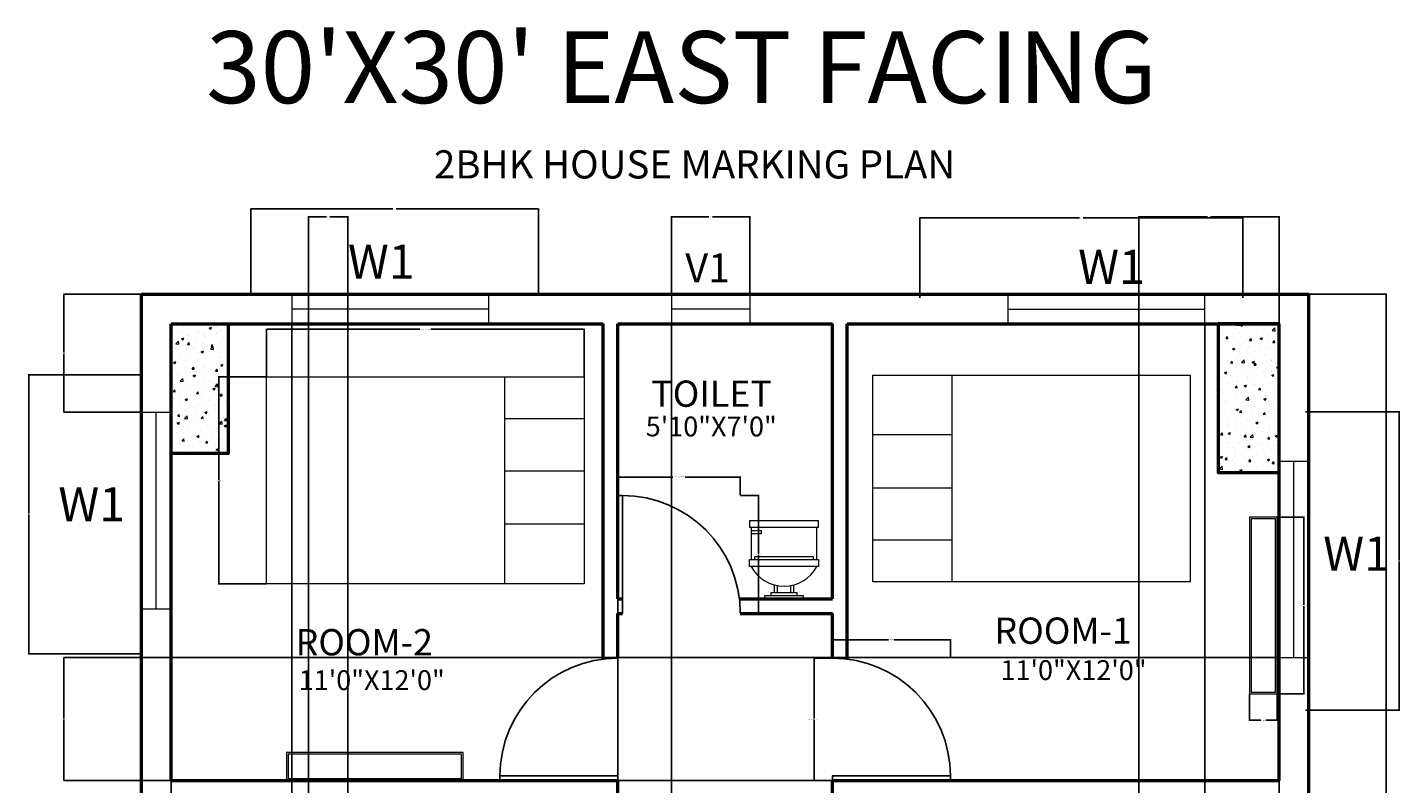
# Model space of a CAD drawing. Units: inches. Extents: x -26 to 394, y -29 to 465.
# Tile 2 of 2: x -25 to 394, y 234 to 465. Entities that reach past the tile are written whole.
import ezdxf

# ---------------------------------------------------------------- set-up
doc = ezdxf.new("R2010")
doc.units = ezdxf.units.IN
doc.header["$MEASUREMENT"] = 0
for name, color, linetype, lineweight, true_color in [('A-ANNO-DIMS', 254, 'Continuous', 18, 0xfeeab9), ('A-COLS', 254, 'Continuous', 50, 0xfeeab9), ('A-COLS-PATT', 31, 'Continuous', 13, 0xfecc66), ('A-FLOR-FIXT', 254, 'Continuous', 18, 0xfeeab9), ('A-FURN', 254, 'Continuous', 18, 0xfeeab9)]:
    doc.layers.add(name, color=color, linetype=linetype, lineweight=lineweight, true_color=true_color)
for name, color, linetype, lineweight in [('A-ANNO-TEXT', 7, 'Continuous', 18), ('A-ANNO-TTLB', 7, 'Continuous', 35), ('A-AREA-IDEN', 7, 'Continuous', 25), ('A-DOOR', 3, 'Continuous', 25), ('A-GLAZ', 4, 'Continuous', 18), ('A-WALL', 7, 'Continuous', 50)]:
    doc.layers.add(name, color=color, linetype=linetype, lineweight=lineweight)
doc.styles.get("Standard").update_dxf_attribs({"font": 'arial.ttf'})
doc.dimstyles.get("Standard").update_dxf_attribs({"dimtxt": 0.18, "dimasz": 0.18, "dimexe": 0.18, "dimexo": 0.0625, "dimgap": 0.09, "dimtad": 0, "dimtih": 1, "dimtoh": 1, "dimdec": 4, "dimzin": 0, "dimdsep": 46, "dimtxsty": 'Standard', "dimcen": 0.09, "dimadec": 0, "dimazin": 0, "dimtfac": 1, "dimtdec": 4, "dimtofl": 0, "dimtmove": 0, "dimatfit": 3, "dimfxl": 1, "dimtolj": 1, "dimtzin": 0, "dimarcsym": 0})

# ---------------------------------------------------------------- blocks, each defined once
blk = doc.blocks.new('*U5')
for p, q in [((-10, 22), (-10, 12)), ((-10, 21), (-7, 21)), ((-7, 21), (-7, 20)), ((10, 12), (10, 22)), ((-7, 20), (-10, 20)), ((9, 13), (-9, 13)), ((-9, 13), (-9, 12)), ((9, 12), (9, 13)), ((10.5, 12), (-10.5, 12)), ((-10.5, 10), (-10.5, 12)), ((10.5, 10), (-10.5, 10)), ((10.5, 12), (10.5, 10)), ((-3, 4.4065), (-3, 2)), ((3, 2), (3, 4.4065)), ((4, 2), (-4, 2)), ((-4, 2), (-4, 1)), ((-2, 2), (-2, 4.1658)), ((2, 4.1658), (2, 2)), ((4, 1), (4, 2))]:
    blk.add_line(p, q)
for points in [[(10.5, 22), (10.5, 24), (-10.5, 24), (-10.5, 22)], [(6, 0), (6, 1), (-6, 1), (-6, 0)]]:
    blk.add_lwpolyline(points, close=True)
blk.add_arc((0, 15.3333), 11.3333, 208.0725, 331.9275)
blk = doc.blocks.new('*D6')
at = {"layer": 'A-ANNO-DIMS', "color": 0, "lineweight": -2, "transparency": 16777216}
for p, q in [((9.23, 358.7), (-24.76, 358.7)), ((-24.58, 358.52), (-24.58, 316.25)), ((-24.58, 273.62), (-24.58, 315.89)), ((9.23, 273.44), (-24.76, 273.44))]:
    blk.add_line(p, q, dxfattribs=at)
at = {"layer": 'A-ANNO-DIMS', "color": 0, "transparency": 16777216}
for points in [[(-24.61, 358.52), (-24.55, 358.52), (-24.58, 358.7)], [(-24.61, 273.62), (-24.55, 273.62), (-24.58, 273.44)]]:
    blk.add_solid(points, dxfattribs=at)
at = {"layer": 'Defpoints', "color": 0, "transparency": 16777216}
for p in [(9.29, 358.7), (-24.58, 273.44), (9.29, 273.44)]:
    blk.add_point(p, dxfattribs=at)
at = {"layer": 'A-ANNO-DIMS', "color": 0, "transparency": 16777216, "insert": (-24.58, 316.07), "char_height": 0.18, "attachment_point": 5}
blk.add_mtext('\\A1;85.2658', dxfattribs=at)
blk = doc.blocks.new('*D7')
at = {"layer": 'A-ANNO-DIMS', "color": 0, "lineweight": -2, "transparency": 16777216}
for p, q in [((43.18, 382.82), (43.18, 409.48)), ((43.36, 409.3), (86.58, 409.3)), ((130.86, 409.3), (87.65, 409.3)), ((131.04, 382.82), (131.04, 409.48))]:
    blk.add_line(p, q, dxfattribs=at)
at = {"layer": 'A-ANNO-DIMS', "color": 0, "transparency": 16777216}
for points in [[(43.36, 409.33), (43.36, 409.27), (43.18, 409.3)], [(130.86, 409.33), (130.86, 409.27), (131.04, 409.3)]]:
    blk.add_solid(points, dxfattribs=at)
at = {"layer": 'Defpoints', "color": 0, "transparency": 16777216}
for p in [(131.04, 409.3), (43.18, 382.76), (131.04, 382.76)]:
    blk.add_point(p, dxfattribs=at)
at = {"layer": 'A-ANNO-DIMS', "color": 0, "transparency": 16777216, "insert": (87.11, 409.3), "char_height": 0.18, "attachment_point": 5}
blk.add_mtext('\\A1;87.8626', dxfattribs=at)
blk = doc.blocks.new('*D8')
at = {"layer": 'A-ANNO-DIMS', "color": 0, "lineweight": -2, "transparency": 16777216}
for p, q in [((247.51, 382.14), (247.51, 406.75)), ((247.69, 406.57), (296.36, 406.57)), ((346.09, 406.57), (297.43, 406.57)), ((346.27, 382.14), (346.27, 406.75))]:
    blk.add_line(p, q, dxfattribs=at)
at = {"layer": 'A-ANNO-DIMS', "color": 0, "transparency": 16777216}
for points in [[(247.69, 406.6), (247.69, 406.54), (247.51, 406.57)], [(346.09, 406.6), (346.09, 406.54), (346.27, 406.57)]]:
    blk.add_solid(points, dxfattribs=at)
at = {"layer": 'Defpoints', "color": 0, "transparency": 16777216}
for p in [(346.27, 406.57), (247.51, 382.08), (346.27, 382.08)]:
    blk.add_point(p, dxfattribs=at)
at = {"layer": 'A-ANNO-DIMS', "color": 0, "transparency": 16777216, "insert": (296.89, 406.57), "char_height": 0.18, "attachment_point": 5}
blk.add_mtext('\\A1;98.7602', dxfattribs=at)
blk = doc.blocks.new('*D9')
at = {"layer": 'A-ANNO-DIMS', "color": 0, "lineweight": -2, "transparency": 16777216}
for p, q in [((365.41, 347.37), (394.13, 347.37)), ((393.95, 347.19), (393.95, 301.96)), ((393.95, 256.37), (393.95, 301.6)), ((365.41, 256.19), (394.13, 256.19))]:
    blk.add_line(p, q, dxfattribs=at)
at = {"layer": 'A-ANNO-DIMS', "color": 0, "transparency": 16777216}
for points in [[(393.92, 347.19), (393.98, 347.19), (393.95, 347.37)], [(393.92, 256.37), (393.98, 256.37), (393.95, 256.19)]]:
    blk.add_solid(points, dxfattribs=at)
at = {"layer": 'Defpoints', "color": 0, "transparency": 16777216}
for p in [(365.34, 347.37), (365.34, 256.19), (393.95, 256.19)]:
    blk.add_point(p, dxfattribs=at)
at = {"layer": 'A-ANNO-DIMS', "color": 0, "transparency": 16777216, "insert": (393.95, 301.78), "char_height": 0.18, "attachment_point": 5}
blk.add_mtext('\\A1;91.1823', dxfattribs=at)
blk = doc.blocks.new('WIN-60IN-9IN-JAMB')
for p, q in [((0, 9), (0, 0)), ((60, 9), (60, 0)), ((0, 4.5), (60, 4.5))]:
    blk.add_line(p, q)
blk = doc.blocks.new('DOOR-36IN-BEDROOM')
blk.add_line((36.04, 1.36), (0.04, 1.36))
blk.add_lwpolyline([(36.04, 1.36), (36.04, 0), (0, 0), (0, 1.36)], close=True)
blk.add_arc((0.04, 1.36), 36, 0, 90)
blk = doc.blocks.new('DOOR-36IN-INTERIOR')
blk.add_lwpolyline([(0, 1.36), (0, 0), (36.04, 0), (36.04, 1.36)], close=True)
blk.add_arc((36, 1.36), 36, 90, 180)
blk = doc.blocks.new('BED-DOUBLE')
for p, q in [((72.74, 63.23), (72.74, 0)), ((72.74, 50.52), (96.99, 50.52)), ((72.74, 34.57), (96.99, 34.57)), ((72.74, 18.32), (96.99, 18.32))]:
    blk.add_line(p, q)
blk.add_lwpolyline([(0, 63.22), (97.03, 63.22), (97.03, 0.09), (0, 0.09)], close=True)
blk = doc.blocks.new('FURN-WALL-UNIT')
for points in [[(8.48, 53.93), (0, 53.93), (0, 0), (8.48, 0)], [(7.98, 53.43), (0.5, 53.43), (0.5, 0.5), (7.98, 0.5)]]:
    blk.add_lwpolyline(points, close=True)
blk = doc.blocks.new('*D20')
at = {"layer": 'A-ANNO-DIMS', "color": 0, "lineweight": -2, "transparency": 16777216}
for p, q in [((356.81, 315.18), (365.02, 315.18)), ((364.84, 315), (364.84, 288.39)), ((364.84, 261.43), (364.84, 288.03)), ((356.81, 261.25), (365.02, 261.25))]:
    blk.add_line(p, q, dxfattribs=at)
at = {"layer": 'A-ANNO-DIMS', "color": 0, "transparency": 16777216}
for points in [[(364.81, 315), (364.87, 315), (364.84, 315.18)], [(364.81, 261.43), (364.87, 261.43), (364.84, 261.25)]]:
    blk.add_solid(points, dxfattribs=at)
at = {"layer": 'Defpoints', "color": 0, "transparency": 16777216}
for p in [(356.75, 315.18), (364.84, 315.18), (356.75, 261.25)]:
    blk.add_point(p, dxfattribs=at)
at = {"layer": 'A-ANNO-DIMS', "color": 0, "transparency": 16777216, "insert": (364.84, 288.21), "char_height": 0.18, "attachment_point": 5}
blk.add_mtext('\\A1;WALL UNIT 53.9288 TYP.', dxfattribs=at)
blk = doc.blocks.new('*D21')
at = {"layer": 'A-ANNO-DIMS', "color": 0, "lineweight": -2, "transparency": 16777216}
for p, q in [((348.26, 261.19), (348.26, 252.98)), ((356.75, 261.19), (356.75, 252.98)), ((348.44, 253.16), (351.73, 253.16)), ((356.57, 253.16), (353.28, 253.16))]:
    blk.add_line(p, q, dxfattribs=at)
at = {"layer": 'A-ANNO-DIMS', "color": 0, "transparency": 16777216}
for points in [[(348.44, 253.19), (348.44, 253.13), (348.26, 253.16)], [(356.57, 253.19), (356.57, 253.13), (356.75, 253.16)]]:
    blk.add_solid(points, dxfattribs=at)
at = {"layer": 'Defpoints', "color": 0, "transparency": 16777216}
for p in [(348.26, 261.25), (356.75, 261.25), (356.75, 253.16)]:
    blk.add_point(p, dxfattribs=at)
at = {"layer": 'A-ANNO-DIMS', "color": 0, "transparency": 16777216, "insert": (352.51, 253.16), "char_height": 0.18, "attachment_point": 5}
blk.add_mtext('\\A1;8.4825 TYP.', dxfattribs=at)
blk = doc.blocks.new('*D22')
at = {"layer": 'A-ANNO-DIMS', "color": 0, "lineweight": -2, "transparency": 16777216}
for p, q in [((220.79, 272.13), (215.07, 272.13)), ((215.25, 271.95), (215.25, 253.64)), ((215.25, 234.95), (215.25, 253.27)), ((220.79, 234.77), (215.07, 234.77))]:
    blk.add_line(p, q, dxfattribs=at)
at = {"layer": 'A-ANNO-DIMS', "color": 0, "transparency": 16777216}
for points in [[(215.22, 271.95), (215.28, 271.95), (215.25, 272.13)], [(215.22, 234.95), (215.28, 234.95), (215.25, 234.77)]]:
    blk.add_solid(points, dxfattribs=at)
at = {"layer": 'Defpoints', "color": 0, "transparency": 16777216}
for p in [(215.25, 272.13), (220.85, 272.13), (220.85, 234.77)]:
    blk.add_point(p, dxfattribs=at)
at = {"layer": 'A-ANNO-DIMS', "color": 0, "transparency": 16777216, "insert": (215.25, 253.45), "char_height": 0.18, "attachment_point": 5}
blk.add_mtext('\\A1;BEDROOM DOOR 37.3627 TYP.', dxfattribs=at)
blk = doc.blocks.new('*D23')
at = {"layer": 'A-ANNO-DIMS', "color": 0, "lineweight": -2, "transparency": 16777216}
for p, q in [((220.85, 272.2), (220.85, 277.92)), ((221.03, 277.74), (238.03, 277.74)), ((256.72, 277.74), (239.72, 277.74)), ((256.9, 272.2), (256.9, 277.92))]:
    blk.add_line(p, q, dxfattribs=at)
at = {"layer": 'A-ANNO-DIMS', "color": 0, "transparency": 16777216}
for points in [[(221.03, 277.77), (221.03, 277.71), (220.85, 277.74)], [(256.72, 277.77), (256.72, 277.71), (256.9, 277.74)]]:
    blk.add_solid(points, dxfattribs=at)
at = {"layer": 'Defpoints', "color": 0, "transparency": 16777216}
for p in [(256.9, 277.74), (220.85, 272.13), (256.9, 272.13)]:
    blk.add_point(p, dxfattribs=at)
at = {"layer": 'A-ANNO-DIMS', "color": 0, "transparency": 16777216, "insert": (238.88, 277.74), "char_height": 0.18, "attachment_point": 5}
blk.add_mtext('\\A1;36.0422 TYP.', dxfattribs=at)
blk = doc.blocks.new('*D24')
at = {"layer": 'A-ANNO-DIMS', "color": 0, "lineweight": -2, "transparency": 16777216}
for p, q in [((155.35, 321.88), (155.35, 327.6)), ((155.53, 327.42), (172.15, 327.42)), ((192.54, 327.42), (175.92, 327.42)), ((192.72, 321.88), (192.72, 327.6))]:
    blk.add_line(p, q, dxfattribs=at)
at = {"layer": 'A-ANNO-DIMS', "color": 0, "transparency": 16777216}
for points in [[(155.53, 327.45), (155.53, 327.39), (155.35, 327.42)], [(192.54, 327.45), (192.54, 327.39), (192.72, 327.42)]]:
    blk.add_solid(points, dxfattribs=at)
at = {"layer": 'Defpoints', "color": 0, "transparency": 16777216}
for p in [(192.72, 327.42), (155.35, 321.81), (192.72, 321.81)]:
    blk.add_point(p, dxfattribs=at)
at = {"layer": 'A-ANNO-DIMS', "color": 0, "transparency": 16777216, "insert": (174.04, 327.42), "char_height": 0.18, "attachment_point": 5}
blk.add_mtext('\\A1;INTERIOR DOOR 37.3627 TYP.', dxfattribs=at)
blk = doc.blocks.new('*D25')
at = {"layer": 'A-ANNO-DIMS', "color": 0, "lineweight": -2, "transparency": 16777216}
for p, q in [((192.78, 321.81), (198.5, 321.81)), ((198.32, 321.63), (198.32, 303.97)), ((198.32, 285.95), (198.32, 303.61)), ((192.78, 285.77), (198.5, 285.77))]:
    blk.add_line(p, q, dxfattribs=at)
at = {"layer": 'A-ANNO-DIMS', "color": 0, "transparency": 16777216}
for points in [[(198.29, 321.63), (198.35, 321.63), (198.32, 321.81)], [(198.29, 285.95), (198.35, 285.95), (198.32, 285.77)]]:
    blk.add_solid(points, dxfattribs=at)
at = {"layer": 'Defpoints', "color": 0, "transparency": 16777216}
for p in [(192.72, 321.81), (192.72, 285.77), (198.32, 285.77)]:
    blk.add_point(p, dxfattribs=at)
at = {"layer": 'A-ANNO-DIMS', "color": 0, "transparency": 16777216, "insert": (198.32, 303.79), "char_height": 0.18, "attachment_point": 5}
blk.add_mtext('\\A1;36.0422 TYP.', dxfattribs=at)
blk = doc.blocks.new('*D28')
at = {"layer": 'A-ANNO-DIMS', "color": 0, "lineweight": -2, "transparency": 16777216}
for p, q in [((47.97, 358.06), (47.97, 372.74)), ((48.15, 372.56), (94.8, 372.56)), ((144.82, 372.56), (98.17, 372.56)), ((145, 358.06), (145, 372.74))]:
    blk.add_line(p, q, dxfattribs=at)
at = {"layer": 'A-ANNO-DIMS', "color": 0, "transparency": 16777216}
for points in [[(48.15, 372.59), (48.15, 372.53), (47.97, 372.56)], [(144.82, 372.59), (144.82, 372.53), (145, 372.56)]]:
    blk.add_solid(points, dxfattribs=at)
at = {"layer": 'Defpoints', "color": 0, "transparency": 16777216}
for p in [(145, 372.56), (47.97, 358), (145, 358)]:
    blk.add_point(p, dxfattribs=at)
at = {"layer": 'A-ANNO-DIMS', "color": 0, "transparency": 16777216, "insert": (96.48, 372.56), "char_height": 0.18, "attachment_point": 5}
blk.add_mtext('\\A1;DOUBLE BED 97.0323 TYP.', dxfattribs=at)
blk = doc.blocks.new('*D29')
at = {"layer": 'A-ANNO-DIMS', "color": 0, "lineweight": -2, "transparency": 16777216}
for p, q in [((47.91, 358), (33.23, 358)), ((33.41, 357.82), (33.41, 326.57)), ((33.41, 294.96), (33.41, 326.21)), ((47.91, 294.78), (33.23, 294.78))]:
    blk.add_line(p, q, dxfattribs=at)
at = {"layer": 'A-ANNO-DIMS', "color": 0, "transparency": 16777216}
for points in [[(33.38, 357.82), (33.44, 357.82), (33.41, 358)], [(33.38, 294.96), (33.44, 294.96), (33.41, 294.78)]]:
    blk.add_solid(points, dxfattribs=at)
at = {"layer": 'Defpoints', "color": 0, "transparency": 16777216}
for p in [(33.41, 358), (47.97, 358), (47.97, 294.78)]:
    blk.add_point(p, dxfattribs=at)
at = {"layer": 'A-ANNO-DIMS', "color": 0, "transparency": 16777216, "insert": (33.41, 326.39), "char_height": 0.18, "attachment_point": 5}
blk.add_mtext('\\A1;63.2256 TYP.', dxfattribs=at)
blk = doc.blocks.new('*D31')
at = {"layer": 'A-ANNO-DIMS', "color": 0, "lineweight": -2, "transparency": 16777216}
for p, q in [((366.42, 383.27), (390.18, 383.27)), ((390, 383.09), (390, 189.45)), ((390, -4.55), (390, 189.09)), ((272.42, -4.73), (390.18, -4.73))]:
    blk.add_line(p, q, dxfattribs=at)
at = {"layer": 'A-ANNO-DIMS', "color": 0, "transparency": 16777216}
for points in [[(389.97, 383.09), (390.03, 383.09), (390, 383.27)], [(389.97, -4.55), (390.03, -4.55), (390, -4.73)]]:
    blk.add_solid(points, dxfattribs=at)
at = {"layer": 'Defpoints', "color": 0, "transparency": 16777216}
for p in [(366.35, 383.27), (390, 383.27), (272.35, -4.73)]:
    blk.add_point(p, dxfattribs=at)
at = {"layer": 'A-ANNO-DIMS', "color": 0, "transparency": 16777216, "insert": (390, 189.27), "char_height": 0.18, "attachment_point": 5}
blk.add_mtext('\\A1;388.0000', dxfattribs=at)
blk = doc.blocks.new('*D33')
at = {"layer": 'A-ANNO-DIMS', "color": 0, "lineweight": -2, "transparency": 16777216}
for p, q in [((171.67, 383.33), (171.67, 407.1)), ((171.85, 406.92), (183.13, 406.92)), ((195.49, 406.92), (184.2, 406.92)), ((195.67, 383.33), (195.67, 407.1))]:
    blk.add_line(p, q, dxfattribs=at)
at = {"layer": 'A-ANNO-DIMS', "color": 0, "transparency": 16777216}
for points in [[(171.85, 406.95), (171.85, 406.89), (171.67, 406.92)], [(195.49, 406.95), (195.49, 406.89), (195.67, 406.92)]]:
    blk.add_solid(points, dxfattribs=at)
at = {"layer": 'Defpoints', "color": 0, "transparency": 16777216}
for p in [(195.67, 406.92), (171.67, 383.27), (195.67, 383.27)]:
    blk.add_point(p, dxfattribs=at)
at = {"layer": 'A-ANNO-DIMS', "color": 0, "transparency": 16777216, "insert": (183.67, 406.92), "char_height": 0.18, "attachment_point": 5}
blk.add_mtext('\\A1;24.0000', dxfattribs=at)
blk = doc.blocks.new('*D34')
at = {"layer": 'A-ANNO-DIMS', "color": 0, "lineweight": -2, "transparency": 16777216}
for p, q in [((155.35, 374.21), (155.35, -28.56)), ((171.67, 374.21), (171.67, -28.56)), ((155.53, -28.38), (162.99, -28.38)), ((171.49, -28.38), (164.04, -28.38))]:
    blk.add_line(p, q, dxfattribs=at)
at = {"layer": 'A-ANNO-DIMS', "color": 0, "transparency": 16777216}
for points in [[(155.53, -28.35), (155.53, -28.41), (155.35, -28.38)], [(171.49, -28.35), (171.49, -28.41), (171.67, -28.38)]]:
    blk.add_solid(points, dxfattribs=at)
at = {"layer": 'Defpoints', "color": 0, "transparency": 16777216}
for p in [(155.35, 374.27), (171.67, 374.27), (171.67, -28.38)]:
    blk.add_point(p, dxfattribs=at)
at = {"layer": 'A-ANNO-DIMS', "color": 0, "transparency": 16777216, "insert": (163.51, -28.38), "char_height": 0.18, "attachment_point": 5}
blk.add_mtext('\\A1;16.3118', dxfattribs=at)
blk = doc.blocks.new('*D35')
at = {"layer": 'A-ANNO-DIMS', "color": 0, "lineweight": -2, "transparency": 16777216}
for p, q in [((314.49, 92.86), (314.49, 407.1)), ((314.67, 406.92), (335.38, 406.92)), ((357.17, 406.92), (336.46, 406.92)), ((357.35, 92.83), (357.35, 407.1))]:
    blk.add_line(p, q, dxfattribs=at)
at = {"layer": 'A-ANNO-DIMS', "color": 0, "transparency": 16777216}
for points in [[(314.67, 406.95), (314.67, 406.89), (314.49, 406.92)], [(357.17, 406.95), (357.17, 406.89), (357.35, 406.92)]]:
    blk.add_solid(points, dxfattribs=at)
at = {"layer": 'Defpoints', "color": 0, "transparency": 16777216}
for p in [(357.35, 406.92), (314.49, 92.8), (357.35, 92.77)]:
    blk.add_point(p, dxfattribs=at)
at = {"layer": 'A-ANNO-DIMS', "color": 0, "transparency": 16777216, "insert": (335.92, 406.92), "char_height": 0.18, "attachment_point": 5}
blk.add_mtext('\\A1;42.8686', dxfattribs=at)
blk = doc.blocks.new('*D36')
at = {"layer": 'A-ANNO-DIMS', "color": 0, "lineweight": -2, "transparency": 16777216}
for p, q in [((18.85, 374.21), (18.85, -28.56)), ((55.78, 374.2), (55.78, -28.56)), ((19.03, -28.38), (36.78, -28.38)), ((55.6, -28.38), (37.85, -28.38))]:
    blk.add_line(p, q, dxfattribs=at)
at = {"layer": 'A-ANNO-DIMS', "color": 0, "transparency": 16777216}
for points in [[(19.03, -28.35), (19.03, -28.41), (18.85, -28.38)], [(55.6, -28.35), (55.6, -28.41), (55.78, -28.38)]]:
    blk.add_solid(points, dxfattribs=at)
at = {"layer": 'Defpoints', "color": 0, "transparency": 16777216}
for p in [(18.85, 374.27), (55.78, 374.27), (55.78, -28.38)]:
    blk.add_point(p, dxfattribs=at)
at = {"layer": 'A-ANNO-DIMS', "color": 0, "transparency": 16777216, "insert": (37.31, -28.38), "char_height": 0.18, "attachment_point": 5}
blk.add_mtext('\\A1;36.9207', dxfattribs=at)
blk = doc.blocks.new('*D37')
at = {"layer": 'A-ANNO-DIMS', "color": 0, "lineweight": -2, "transparency": 16777216}
for p, q in [((334.57, 374.05), (334.57, -28.56)), ((357.35, 374.21), (357.35, -28.56)), ((334.75, -28.38), (345.43, -28.38)), ((357.17, -28.38), (346.5, -28.38))]:
    blk.add_line(p, q, dxfattribs=at)
at = {"layer": 'A-ANNO-DIMS', "color": 0, "transparency": 16777216}
for points in [[(334.75, -28.35), (334.75, -28.41), (334.57, -28.38)], [(357.17, -28.35), (357.17, -28.41), (357.35, -28.38)]]:
    blk.add_solid(points, dxfattribs=at)
at = {"layer": 'Defpoints', "color": 0, "transparency": 16777216}
for p in [(334.57, 374.11), (357.35, 374.27), (357.35, -28.38)]:
    blk.add_point(p, dxfattribs=at)
at = {"layer": 'A-ANNO-DIMS', "color": 0, "transparency": 16777216, "insert": (345.96, -28.38), "char_height": 0.18, "attachment_point": 5}
blk.add_mtext('\\A1;22.7852', dxfattribs=at)
blk = doc.blocks.new('*D38')
at = {"layer": 'A-ANNO-DIMS', "color": 0, "lineweight": -2, "transparency": 16777216}
for p, q in [((9.79, 383.27), (-14.04, 383.27)), ((-13.86, 383.09), (-13.86, 365.43)), ((-13.86, 347.4), (-13.86, 365.06)), ((9.73, 347.22), (-14.04, 347.22))]:
    blk.add_line(p, q, dxfattribs=at)
at = {"layer": 'A-ANNO-DIMS', "color": 0, "transparency": 16777216}
for points in [[(-13.89, 383.09), (-13.83, 383.09), (-13.86, 383.27)], [(-13.89, 347.4), (-13.83, 347.4), (-13.86, 347.22)]]:
    blk.add_solid(points, dxfattribs=at)
at = {"layer": 'Defpoints', "color": 0, "transparency": 16777216}
for p in [(9.85, 383.27), (-13.86, 347.22), (9.79, 347.22)]:
    blk.add_point(p, dxfattribs=at)
at = {"layer": 'A-ANNO-DIMS', "color": 0, "transparency": 16777216, "insert": (-13.86, 365.25), "char_height": 0.18, "attachment_point": 5}
blk.add_mtext('\\A1;36.0512', dxfattribs=at)
blk = doc.blocks.new('*D40')
at = {"layer": 'A-ANNO-DIMS', "color": 0, "lineweight": -2, "transparency": 16777216}
for p, q in [((357.24, 272.29), (-14.04, 272.29)), ((-13.86, 272.11), (-13.86, 253.71)), ((-13.86, 234.95), (-13.86, 253.35)), ((357.29, 234.77), (-14.04, 234.77))]:
    blk.add_line(p, q, dxfattribs=at)
at = {"layer": 'A-ANNO-DIMS', "color": 0, "transparency": 16777216}
for points in [[(-13.89, 272.11), (-13.83, 272.11), (-13.86, 272.29)], [(-13.89, 234.95), (-13.83, 234.95), (-13.86, 234.77)]]:
    blk.add_solid(points, dxfattribs=at)
at = {"layer": 'Defpoints', "color": 0, "transparency": 16777216}
for p in [(-13.86, 272.29), (357.3, 272.29), (357.35, 234.77)]:
    blk.add_point(p, dxfattribs=at)
at = {"layer": 'A-ANNO-DIMS', "color": 0, "transparency": 16777216, "insert": (-13.86, 253.53), "char_height": 0.18, "attachment_point": 5}
blk.add_mtext('\\A1;37.5215', dxfattribs=at)
blk = doc.blocks.new('*D42')
at = {"layer": 'A-ANNO-DIMS', "color": 0, "lineweight": -2, "transparency": 16777216}
for p, q in [((60.85, 73.33), (60.85, 407.1)), ((61.03, 406.92), (66.33, 406.92)), ((72.67, 406.92), (67.38, 406.92)), ((72.85, 73.33), (72.85, 407.1))]:
    blk.add_line(p, q, dxfattribs=at)
at = {"layer": 'A-ANNO-DIMS', "color": 0, "transparency": 16777216}
for points in [[(61.03, 406.95), (61.03, 406.89), (60.85, 406.92)], [(72.67, 406.95), (72.67, 406.89), (72.85, 406.92)]]:
    blk.add_solid(points, dxfattribs=at)
at = {"layer": 'Defpoints', "color": 0, "transparency": 16777216}
for p in [(72.85, 406.92), (60.85, 73.27), (72.85, 73.27)]:
    blk.add_point(p, dxfattribs=at)
at = {"layer": 'A-ANNO-DIMS', "color": 0, "transparency": 16777216, "insert": (66.85, 406.92), "char_height": 0.18, "attachment_point": 5}
blk.add_mtext('\\A1;12.0000', dxfattribs=at)

msp = doc.modelspace()

# ---------------------------------------------------------------- hatches: boundary and pattern name
at = {"layer": 'A-COLS-PATT'}
h = msp.add_hatch(dxfattribs=at)
h.set_pattern_fill('AR-CONC', color=256)
h.paths.add_polyline_path([(36.3265, 374.27084), (18.85458, 374.27084), (18.85458, 334.60955), (36.3265, 334.60955)])
h = msp.add_hatch(dxfattribs=at)
h.set_pattern_fill('AR-CONC', color=256)
h.set_pattern_definition([(50, (0, 0), (7.1726, -0.62752), [0.75, -8.25]), (355, (0, 0), (-1.38751, 7.52192), [0.6, -6.6]), (100.4514, (0.598, -0.052), (5.78509, 6.8944), [0.6374, -7.01142]), (46.1842, (0, 2), (10.67241, -1.6552), [1.125, -12.375]), (96.6356, (0.889, 1.862), (9.34662, 9.74119), [0.9561, -10.51714]), (351.1842, (0, 2), (9.34662, 9.74119), [0.9, -9.9]), (21, (1, 1.5), (5.96907, -4.02619), [0.75, -8.25]), (326, (1, 1.5), (2.43315, 7.2515), [0.6, -6.6]), (71.4514, (1.4974, 1.1645), (8.40222, 3.22531), [0.6374, -7.01142]), (37.5, (0, 0), (0.121599, 3.328939), [0, -6.52, 0, -6.7, 0, -6.625]), (7.5, (0, 0), (2.630695, 3.944117), [0, -3.82, 0, -6.37, 0, -2.525]), (327.5, (-2.23, 0), (5.338224, -0.225549), [0, -2.5, 0, -7.8, 0, -10.35]), (317.5, (-3.23, 0), (5.83186, 1.00105), [0, -3.25, 0, -5.18, 0, -7.35])])
h.paths.add_polyline_path([(338.70558, 374.27084), (338.70558, 328.84584), (357.35458, 328.84584), (357.35458, 374.27084)])

# ---------------------------------------------------------------- linework, layer by layer
at = {"layer": 'A-COLS'}
for points in [[(18.85458, 374.27084), (36.3265, 374.27084), (36.3265, 334.60955), (18.85458, 334.60955)], [(18.85458, 374.27084), (36.3265, 374.27084), (36.3265, 334.60955), (18.85458, 334.60955)], [(357.35458, 374.27084), (338.70558, 374.27084), (338.70558, 328.84584), (357.35458, 328.84584)]]:
    msp.add_lwpolyline(points, close=True, dxfattribs=at)
at = {"layer": 'A-FURN'}
msp.add_lwpolyline([(107.5733, 235.3196), (107.5733, 242.80209), (54.6445, 242.80209), (54.6445, 235.3196)], close=True, dxfattribs=at)
at = {"layer": 'A-GLAZ'}
for p, q in [((171.66634, 383.27148), (171.66634, 374.27148)), ((195.66634, 383.27148), (195.66634, 374.27148)), ((171.66634, 378.77148), (195.66634, 378.77148))]:
    msp.add_line(p, q, dxfattribs=at)
at = {"layer": 'A-WALL'}
for p, q in [((9.85458, 4.27084), (9.85458, 383.27084)), ((9.85458, 383.27084), (366.35458, 383.27084)), ((366.35458, 88.27084), (366.35458, 383.27084)), ((18.85458, 374.27084), (150.85458, 374.27084)), ((18.85458, 234.77084), (18.85458, 374.27084)), ((150.85458, 271.85645), (150.85458, 374.27084)), ((155.35458, 374.27084), (220.85458, 374.27084)), ((155.35458, 290.27084), (155.35458, 374.27084)), ((220.85458, 290.27084), (220.85458, 374.27084)), ((225.35458, 271.85645), (225.35458, 374.27084)), ((225.35458, 374.27084), (357.35458, 374.27084)), ((357.35458, 234.77084), (357.35458, 374.27084)), ((155.35458, 290.27084), (156.71727, 290.27084)), ((192.4402, 290.27084), (220.85458, 290.27084)), ((155.35458, 285.77084), (156.71727, 285.77084)), ((155.35458, 272.1335), (155.35458, 285.77084)), ((192.71724, 285.77084), (220.85458, 285.77084)), ((220.85458, 272.1335), (220.85458, 285.77084)), ((18.85458, 234.77084), (155.35458, 234.77084)), ((150.85458, 234.77084), (150.85458, 234.84244)), ((155.35458, 230.27084), (155.35458, 234.77084)), ((220.85458, 234.77084), (357.35458, 234.77084)), ((220.85458, 230.27084), (220.85458, 234.77084))]:
    msp.add_line(p, q, dxfattribs=at)

# ---------------------------------------------------------------- block references
at = {"layer": 'A-DOOR', "rotation": 269.9999999999999}
msp.add_blockref('DOOR-36IN-INTERIOR', (155.35458, 321.813), dxfattribs=at)
at = {"layer": 'A-DOOR', "extrusion": (0, 0, -1), "zscale": -1}
msp.add_blockref('DOOR-36IN-BEDROOM', (-155.35458, 234.77084), dxfattribs=at)
at = {"layer": 'A-DOOR'}
msp.add_blockref('DOOR-36IN-BEDROOM', (220.85458, 234.77084), dxfattribs=at)
at = {"layer": 'A-FLOR-FIXT'}
msp.add_blockref('*U5', (206.07263, 290.10378), dxfattribs=at)
at = {"layer": 'A-FURN'}
for name, p in [('BED-DOUBLE', (47.96763, 294.7763)), ('FURN-WALL-UNIT', (348.26482, 261.24755))]:
    msp.add_blockref(name, p, dxfattribs=at)
for name, p, rotation in [('BED-DOUBLE', (330.18399, 358.62408), 180), ('FURN-WALL-UNIT', (54.1445, 243.30209), 269.9999999999999)]:
    msp.add_blockref(name, p, dxfattribs=dict(at, rotation=rotation))
at = {"layer": 'A-GLAZ'}
msp.add_blockref('WIN-60IN-9IN-JAMB', (55.77527, 374.26724), dxfattribs=at)
for p, rotation in [((334.56939, 383.11204), 180), ((18.79028, 287.21962), 90.0000000000001), ((366.29877, 272.29231), 90.0000000000001)]:
    msp.add_blockref('WIN-60IN-9IN-JAMB', p, dxfattribs=dict(at, rotation=rotation))

# ---------------------------------------------------------------- texts
at = {"layer": 'A-ANNO-TEXT'}
for s, height, p in [('W1', 10.431092, (72.85688, 388.00648)), ('V1', 8.857947, (175.92507, 386.85827)), ('W1', 10.431092, (295.90998, 386.40201)), ('W1', 10.431092, (-15.5939, 313.89713)), ('W1', 10.431092, (370.77816, 298.82104))]:
    msp.add_text(s, height=height, dxfattribs=at).set_placement(p)
at = {"layer": 'A-ANNO-TTLB'}
for s, height, p in [("30'X30' EAST FACING", 21.9633072, (29.567, 441.64062)), ('2BHK HOUSE MARKING PLAN', 8.6144341, (99.15325, 418.61551))]:
    msp.add_text(s, height=height, dxfattribs=at).set_placement(p)
at = {"layer": 'A-AREA-IDEN'}
for s, height, p in [('TOILET', 8.023641, (165.52511, 348.88095)), ('5\'10"X7\'0"', 6.048069, (163.83822, 339.84672)), ('ROOM-2', 8.023641, (56.87663, 272.96833)), ('ROOM-1', 8.023641, (270.35069, 276.49648)), ('11\'0"X12\'0"', 6.0480693, (57.84234, 262.38217)), ('11\'0"X12\'0"', 6.0480693, (272.20291, 265.44602))]:
    msp.add_text(s, height=height, dxfattribs=at).set_placement(p)

# ---------------------------------------------------------------- dimensions: what is measured, and where the dimension line sits
at = {"layer": 'A-ANNO-DIMS'}
for base, p1, p2, override, picture, middle in [((131.04342, 409.29532), (43.18084, 382.75719), (131.04342, 382.75719), {"dimclrd": 0, "dimclre": 0, "dimclrt": 0}, '*D7', (87.11213, 409.29532)), ((72.85459, 406.92148), (60.85459, 73.27084), (72.85459, 73.27084), {"dimdec": 4, "dimlfac": 1, "dimrnd": 0, "dimzin": 0, "dimdsep": 46, "dimlunit": 2}, '*D42', (66.85459, 406.92148)), ((195.66634, 406.92148), (171.66634, 383.27148), (195.66634, 383.27148), {"dimdec": 4, "dimlfac": 1, "dimrnd": 0, "dimzin": 0, "dimdsep": 46, "dimlunit": 2}, '*D33', (183.66634, 406.92148)), ((357.354585, 406.921485), (314.486028, 92.797666), (357.354585, 92.770839), {"dimdec": 4, "dimlfac": 1, "dimrnd": 0, "dimzin": 0, "dimdsep": 46, "dimlunit": 2}, '*D35', (335.920306, 406.921485)), ((346.27268, 406.57346), (247.51244, 382.07676), (346.27268, 382.07676), {"dimclrd": 0, "dimclre": 0, "dimclrt": 0}, '*D8', (296.89256, 406.57346)), ((55.77527, -28.37916), (18.85458, 374.27084), (55.77527, 374.26724), {"dimdec": 4, "dimlfac": 1, "dimrnd": 0, "dimzin": 0, "dimdsep": 46, "dimlunit": 2}, '*D36', (37.31493, -28.37916)), ((171.66634, -28.37916), (155.35458, 374.27084), (171.66634, 374.27148), {"dimdec": 4, "dimlfac": 1, "dimrnd": 0, "dimzin": 0, "dimdsep": 46, "dimlunit": 2}, '*D34', (163.51046, -28.37916)), ((357.35458, -28.37916), (334.56939, 374.11204), (357.35458, 374.27084), {"dimdec": 4, "dimlfac": 1, "dimrnd": 0, "dimzin": 0, "dimdsep": 46, "dimlunit": 2}, '*D37', (345.96199, -28.37916))]:
    dim = msp.add_linear_dim(base=base, p1=p1, p2=p2, dimstyle='Standard', override=override, dxfattribs=at)
    dim.commit()
    dim.dimension.update_dxf_attribs({"geometry": picture, "text_midpoint": middle})
for base, p1, p2, override, picture, middle in [((-13.85972, 347.21962), (9.85458, 383.27084), (9.79028, 347.21962), {"dimdec": 4, "dimlfac": 1, "dimrnd": 0, "dimzin": 0, "dimdsep": 46, "dimlunit": 2}, '*D38', (-13.85972, 365.24523)), ((390.00459, 383.27084), (272.35458, -4.72916), (366.35458, 383.27084), {"dimdec": 4, "dimlfac": 1, "dimrnd": 0, "dimzin": 0, "dimdsep": 46, "dimlunit": 2}, '*D31', (390.00459, 189.27084)), ((-24.57529, 273.43659), (9.29213, 358.70236), (9.29213, 273.43659), {"dimclrd": 0, "dimclre": 0, "dimclrt": 0}, '*D6', (-24.57529, 316.06948)), ((393.94991, 256.19079), (365.34348, 347.37305), (365.34348, 256.19079), {"dimclrd": 0, "dimclre": 0, "dimclrt": 0}, '*D9', (393.94991, 301.78192)), ((-13.85972, 272.29231), (357.35458, 234.77084), (357.29877, 272.29231), {"dimdec": 4, "dimlfac": 1, "dimrnd": 0, "dimzin": 0, "dimdsep": 46, "dimlunit": 2}, '*D40', (-13.85972, 253.53157))]:
    dim = msp.add_linear_dim(base=base, p1=p1, p2=p2, angle=90, dimstyle='Standard', override=override, dxfattribs=at)
    dim.commit()
    dim.dimension.update_dxf_attribs({"geometry": picture, "text_midpoint": middle})
for base, p1, p2, text, picture, middle in [((144.9999, 372.55677), (47.96763, 358.00193), (144.9999, 358.00193), 'DOUBLE BED <> TYP.', '*D28', (96.48377, 372.55677)), ((192.71727, 327.4174), (155.35458, 321.813), (192.71727, 321.813), 'INTERIOR DOOR <> TYP.', '*D24', (174.03593, 327.4174)), ((256.89674, 277.73792), (220.85458, 272.13352), (256.89674, 272.13352), '<> TYP.', '*D23', (238.87566, 277.73792)), ((356.74731, 253.15823), (348.26482, 261.24755), (356.74731, 261.24755), '<> TYP.', '*D21', (352.50606, 253.15823))]:
    dim = msp.add_linear_dim(base=base, p1=p1, p2=p2, text=text, dimstyle='Standard', override={"dimdec": 4, "dimlfac": 1, "dimrnd": 0, "dimzin": 0, "dimdsep": 46, "dimlunit": 2}, dxfattribs=at)
    dim.commit()
    dim.dimension.update_dxf_attribs({"geometry": picture, "text_midpoint": middle})
for base, p1, p2, angle, text, picture, middle in [((33.41279, 358.00193), (47.96763, 294.7763), (47.96763, 358.00193), 90, '<> TYP.', '*D29', (33.41279, 326.38911)), ((198.32167, 285.77084), (192.71727, 321.813), (192.71727, 285.77084), 270, '<> TYP.', '*D25', (198.32167, 303.79192)), ((364.83663, 315.17636), (356.74731, 261.24755), (356.74731, 315.17636), 90, 'WALL UNIT <> TYP.', '*D20', (364.83663, 288.21196)), ((215.25018, 272.13352), (220.85458, 234.77084), (220.85458, 272.13352), 90, 'BEDROOM DOOR <> TYP.', '*D22', (215.25018, 253.45218))]:
    dim = msp.add_linear_dim(base=base, p1=p1, p2=p2, angle=angle, text=text, dimstyle='Standard', override={"dimdec": 4, "dimlfac": 1, "dimrnd": 0, "dimzin": 0, "dimdsep": 46, "dimlunit": 2}, dxfattribs=at)
    dim.commit()
    dim.dimension.update_dxf_attribs({"geometry": picture, "text_midpoint": middle})

doc.saveas('drawing.dxf')
